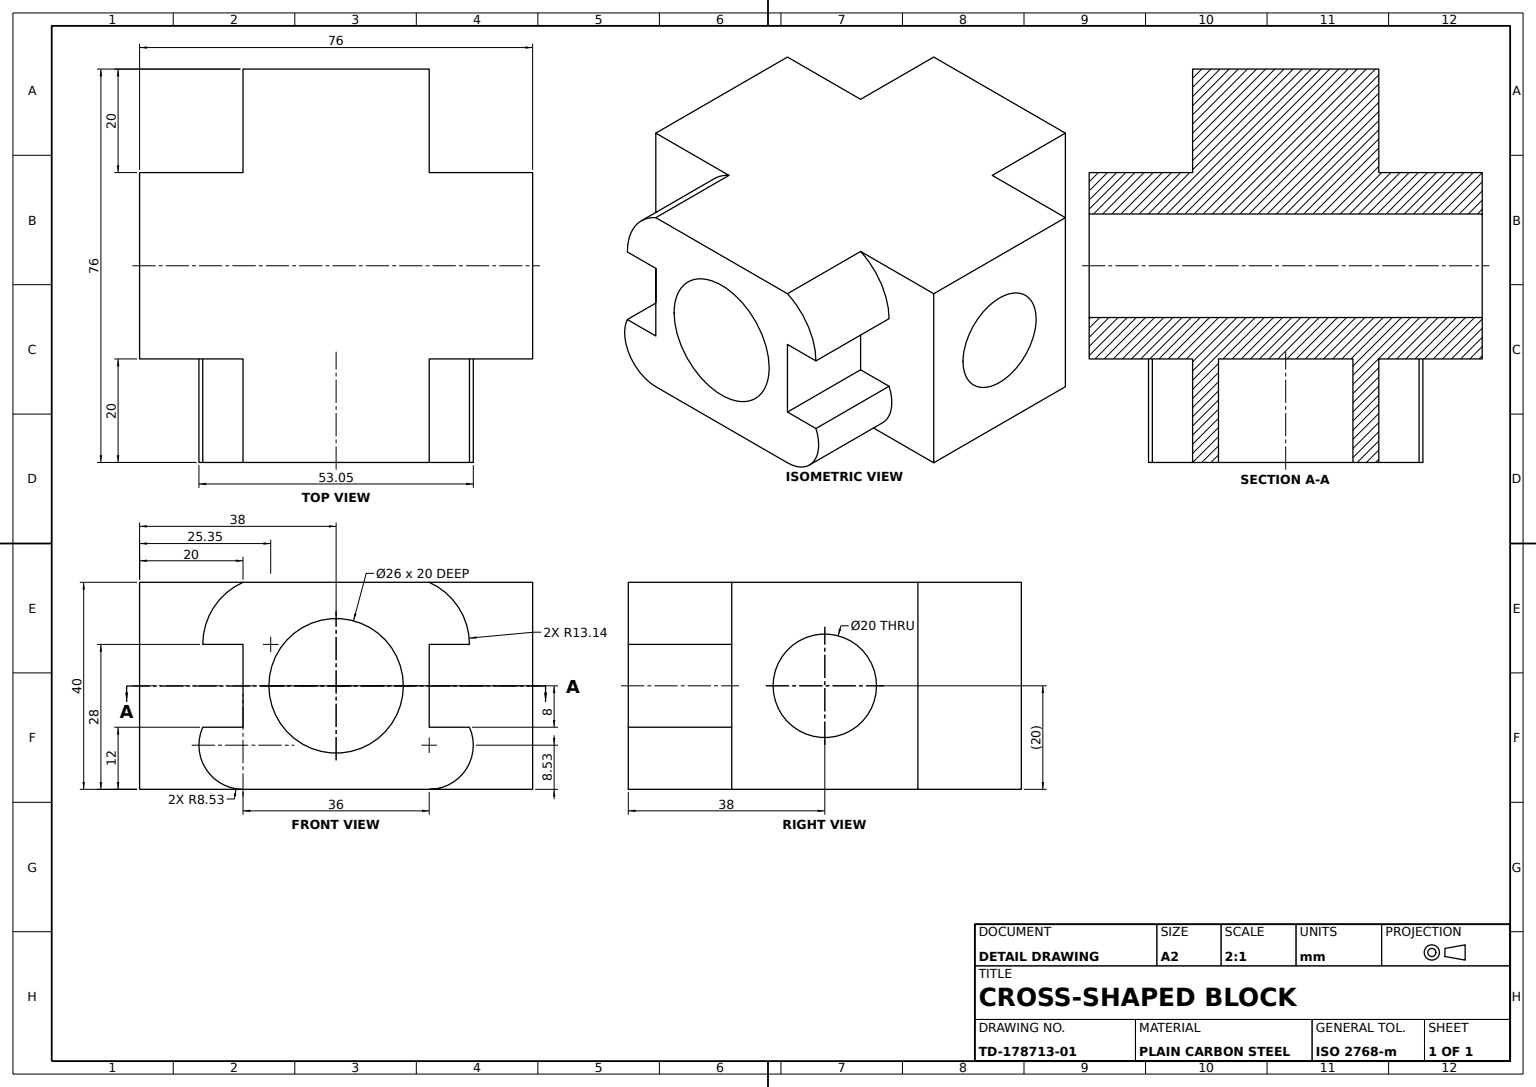
SolidWorks part; units mm, degrees
material "Plain Carbon Steel"
ref_plane "Front Plane" through (0, 0, 0) normal (0, 0, 1) x (1, 0, 0)
ref_plane "Top Plane" through (0, 0, 0) normal (0, 1, 0) x (1, 0, 0)
ref_plane "Right Plane" through (0, 0, 0) normal (1, 0, 0) x (0, 0, -1)
sketch "Cross Profile Sketch" plane through (0, 0, 0) normal (0, 1, 0) x (1, 0, 0)
  line L0 (0, 0) -> (20, 0)
  line L1 (20, 0) -> (20, 20)
  line L2 (20, 20) -> (56, 20)
  line L3 (56, 20) -> (56, 0)
  line L4 (56, 0) -> (76, 0)
  line L5 (76, 0) -> (76, -36)
  line L6 (76, -36) -> (56, -36)
  line L7 (56, -36) -> (56, -56)
  line L8 (56, -56) -> (20, -56)
  line L9 (20, -56) -> (20, -36)
  line L10 (20, -36) -> (0, -36)
  line L11 (0, -36) -> (0, 0)
  dimension "D1" = 36
  dimension "D2" = 36
  dimension "D3" = 36
  dimension "D4" = 36
  dimension "D5" = 20
  dimension "D6" = 20
  dimension "D7" = 20
  dimension "D8" = 20
  dimension "D9" = 20
extrude "Cross Block" add sketch "Cross Profile Sketch" along normal blind 40
sketch "Side Lug Sketch" plane through (0, 0, 56) normal (0, 0, 1) x (1, 0, 0)
  line L0 (38, 40) -> (38, 0) construction
  line L1 (20, 40) -> (56, 40) construction
  line L2 (20, 0) -> (56, 0) construction
  line L3 (38, 20) -> (38, 28)
  line L4 (48.247, 28) -> (63.7876, 28)
  line L5 (27.753, 28) -> (12.2124, 28)
  line L6 (38, 20) -> (38, 12)
  line L7 (48.247, 12) -> (63.7876, 12)
  line L8 (27.753, 12) -> (12.2124, 12)
  line L9 (20, 40) -> (56, 40)
  line L10 (56, 0) -> (20, 0)
  arc A1 (27.753, 12) -> (48.247, 12) centre (38, 20) ccw
  arc A2 (48.247, 28) -> (27.753, 28) centre (38, 20) ccw
  arc A4 (20, 0) -> (12.2124, 12) centre (20, 8.5269) cw
  arc A5 (56, 0) -> (63.7876, 12) centre (56, 8.5269) ccw
  arc A6 (12.2124, 28) -> (20, 40) centre (25.3517, 28) cw
  arc A7 (63.7876, 28) -> (56, 40) centre (50.6483, 28) ccw
  line M19 (56, 0) -> (56, 40)
  line M21 (20, 40) -> (20, 0)
  dimension "D1" = 13.1393
  dimension "D2" = 26
  dimension "D5" = 8.5269
  dimension "D6" = 16
  dimension "D7" = 8.5269
  dimension "D8" = 13.1393
  dimension "D3" = 8
  dimension "D4" = 8
extrude "Side Lug" add sketch "Side Lug Sketch" against normal blind 20 contours A6 L5 M21 | L4 A7 M19 | A5 L7 M19 | A4 L8 M21
sketch "Bore Ø26 Sketch" plane through (0, 0, 56) normal (0, 0, 1) x (1, 0, 0)
  line L0 (38, 40) -> (38, 0) construction
  line L1 (20, 40) -> (56, 40) construction
  line L2 (20, 0) -> (56, 0) construction
  circle A0 centre (38, 20) radius 13
  dimension "D1" = 26
extrude "Bore Ø26" cut sketch "Bore Ø26 Sketch" against normal blind 20
sketch "Cross Hole Ø20 Sketch" plane through (76, 0, 0) normal (1, 0, 0) x (0, 0, -1)
  line L0 (-18, 40) -> (-18, 0) construction
  line L1 (-36, 40) -> (0, 40) construction
  line L2 (-36, 0) -> (0, 0) construction
  circle A0 centre (-18, 20) radius 10
  dimension "D1" = 20
extrude "Cross Hole Ø20" cut sketch "Cross Hole Ø20 Sketch" against normal through all
